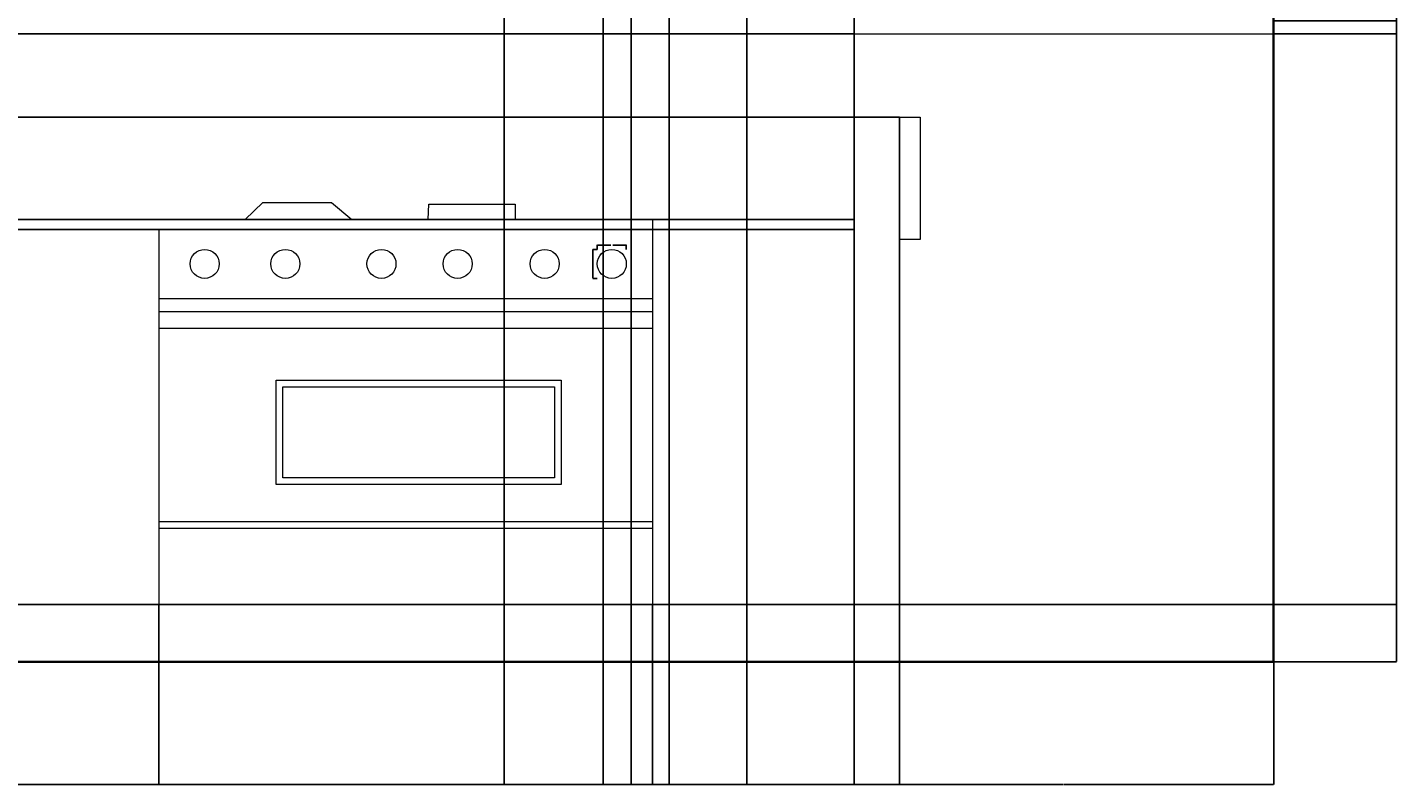
# Model space of a CAD drawing. Units: millimetres. Extents: x 4725 to 8727, y 2935 to 5260.
# Tile 2 of 3: x 6642 to 8727, y 2935 to 4087. Entities that reach past the tile are written whole.
import ezdxf

# ---------------------------------------------------------------- set-up
doc = ezdxf.new("R2010")
doc.units = ezdxf.units.MM
for name, color, linetype, lineweight in [('A-ANNO-DIMS', 2, 'Continuous', 18), ('A-CASE-CTOP', 7, 'Continuous', 25), ('A-ELEV', 7, 'Continuous', 35), ('A-EQPM', 4, 'Continuous', 18), ('A-FLOR-CASE', 8, 'Continuous', 25)]:
    doc.layers.add(name, color=color, linetype=linetype, lineweight=lineweight)
doc.styles.get("Standard").update_dxf_attribs({"font": 'arial.ttf'})
doc.dimstyles.get("Standard").update_dxf_attribs({"dimtxt": 0.18, "dimasz": 0.18, "dimexe": 0.18, "dimexo": 0.0625, "dimgap": 0.09, "dimtad": 0, "dimtih": 1, "dimtoh": 1, "dimdec": 4, "dimzin": 0, "dimdsep": 46, "dimtxsty": 'Standard', "dimcen": 0.09, "dimadec": 0, "dimazin": 0, "dimtfac": 1, "dimtdec": 4, "dimtofl": 0, "dimtmove": 0, "dimatfit": 3, "dimfxl": 1, "dimtolj": 1, "dimtzin": 0, "dimarcsym": 0})

# ---------------------------------------------------------------- blocks, each defined once
blk = doc.blocks.new('REFRIGERATOR-DOOR-PULL')
blk.add_lwpolyline([(0, 186.1), (31.3, 186.1), (31.3, 0), (0, 0)], close=True)
blk = doc.blocks.new('COOKER-CONTROL-KNOB')
blk.add_circle((22.1, 22.1), 22.1)
blk = doc.blocks.new('*D3')
at = {"layer": 'A-ANNO-DIMS', "color": 0, "lineweight": -2, "transparency": 16777216}
for p, q in [((7509.7, 3749.5), (7509.7, 3756.3)), ((7509.8, 3756.1), (7530.3, 3756.1)), ((7553.7, 3756.1), (7533.3, 3756.1)), ((7553.8, 3749.5), (7553.8, 3756.3))]:
    blk.add_line(p, q, dxfattribs=at)
at = {"layer": 'A-ANNO-DIMS', "color": 0, "transparency": 16777216}
for points in [[(7509.8, 3756.1), (7509.8, 3756), (7509.7, 3756.1)], [(7553.7, 3756.1), (7553.7, 3756), (7553.8, 3756.1)]]:
    blk.add_solid(points, dxfattribs=at)
at = {"layer": 'Defpoints', "color": 0, "transparency": 16777216}
for p in [(7553.8, 3756.1), (7509.7, 3749.4), (7553.8, 3749.4)]:
    blk.add_point(p, dxfattribs=at)
at = {"layer": 'A-ANNO-DIMS', "color": 0, "transparency": 16777216, "insert": (7531.8, 3756.1), "char_height": 0.18, "attachment_point": 5}
blk.add_mtext('\\A1;COOKER KNOB 44 TYP.', dxfattribs=at)
blk = doc.blocks.new('*D4')
at = {"layer": 'A-ANNO-DIMS', "color": 0, "lineweight": -2, "transparency": 16777216}
for p, q in [((7509.6, 3749.4), (7502.9, 3749.4)), ((7503, 3749.3), (7503, 3727.5)), ((7503, 3705.4), (7503, 3727.2)), ((7509.6, 3705.3), (7502.9, 3705.3))]:
    blk.add_line(p, q, dxfattribs=at)
at = {"layer": 'A-ANNO-DIMS', "color": 0, "transparency": 16777216}
for points in [[(7503, 3749.3), (7503.1, 3749.3), (7503, 3749.4)], [(7503, 3705.4), (7503.1, 3705.4), (7503, 3705.3)]]:
    blk.add_solid(points, dxfattribs=at)
at = {"layer": 'Defpoints', "color": 0, "transparency": 16777216}
for p in [(7503, 3749.4), (7509.7, 3749.4), (7509.7, 3705.3)]:
    blk.add_point(p, dxfattribs=at)
at = {"layer": 'A-ANNO-DIMS', "color": 0, "transparency": 16777216, "insert": (7503, 3727.4), "char_height": 0.18, "attachment_point": 5}
blk.add_mtext('\\A1;44 TYP.', dxfattribs=at)
blk = doc.blocks.new('*D10')
at = {"layer": 'A-ANNO-DIMS', "color": 0, "lineweight": -2, "transparency": 16777216}
for p, q in [((6031.8, 3209), (6031.8, 2934.7)), ((6841.9, 3209), (6841.9, 2934.7)), ((6032, 2934.8), (6436.5, 2934.8)), ((6841.8, 2934.8), (6437.3, 2934.8))]:
    blk.add_line(p, q, dxfattribs=at)
at = {"layer": 'A-ANNO-DIMS', "color": 0, "transparency": 16777216}
for points in [[(6032, 2934.9), (6032, 2934.8), (6031.8, 2934.8)], [(6841.8, 2934.9), (6841.8, 2934.8), (6841.9, 2934.8)]]:
    blk.add_solid(points, dxfattribs=at)
at = {"layer": 'Defpoints', "color": 0, "transparency": 16777216}
for p in [(6031.8, 3209), (6841.9, 3209), (6841.9, 2934.8)]:
    blk.add_point(p, dxfattribs=at)
at = {"layer": 'A-ANNO-DIMS', "color": 0, "transparency": 16777216, "insert": (6436.9, 2934.8), "char_height": 0.18, "attachment_point": 5}
blk.add_mtext('\\A1;810.2', dxfattribs=at)
blk = doc.blocks.new('*D11')
at = {"layer": 'A-ANNO-DIMS', "color": 0, "lineweight": -2, "transparency": 16777216}
for p, q in [((6841.9, 3209), (6841.9, 2934.7)), ((7593.8, 3209), (7593.8, 2934.7)), ((6842.1, 2934.8), (7217.5, 2934.8)), ((7593.6, 2934.8), (7218.3, 2934.8))]:
    blk.add_line(p, q, dxfattribs=at)
at = {"layer": 'A-ANNO-DIMS', "color": 0, "transparency": 16777216}
for points in [[(6842.1, 2934.9), (6842.1, 2934.8), (6841.9, 2934.8)], [(7593.6, 2934.9), (7593.6, 2934.8), (7593.8, 2934.8)]]:
    blk.add_solid(points, dxfattribs=at)
at = {"layer": 'Defpoints', "color": 0, "transparency": 16777216}
for p in [(6841.9, 3209), (7593.8, 3209), (7593.8, 2934.8)]:
    blk.add_point(p, dxfattribs=at)
at = {"layer": 'A-ANNO-DIMS', "color": 0, "transparency": 16777216, "insert": (7217.9, 2934.8), "char_height": 0.18, "attachment_point": 5}
blk.add_mtext('\\A1;751.9', dxfattribs=at)
blk = doc.blocks.new('*D12')
at = {"layer": 'A-ANNO-DIMS', "color": 0, "lineweight": -2, "transparency": 16777216}
for p, q in [((7593.8, 3209), (7593.8, 2934.7)), ((7900.9, 3121.6), (7900.9, 2934.7)), ((7594, 2934.8), (7746.9, 2934.8)), ((7900.7, 2934.8), (7747.8, 2934.8))]:
    blk.add_line(p, q, dxfattribs=at)
at = {"layer": 'A-ANNO-DIMS', "color": 0, "transparency": 16777216}
for points in [[(7594, 2934.9), (7594, 2934.8), (7593.8, 2934.8)], [(7900.7, 2934.9), (7900.7, 2934.8), (7900.9, 2934.8)]]:
    blk.add_solid(points, dxfattribs=at)
at = {"layer": 'Defpoints', "color": 0, "transparency": 16777216}
for p in [(7593.8, 3209), (7900.9, 3121.7), (7900.9, 2934.8)]:
    blk.add_point(p, dxfattribs=at)
at = {"layer": 'A-ANNO-DIMS', "color": 0, "transparency": 16777216, "insert": (7747.3, 2934.8), "char_height": 0.18, "attachment_point": 5}
blk.add_mtext('\\A1;307.04', dxfattribs=at)
blk = doc.blocks.new('*D13')
at = {"layer": 'A-ANNO-DIMS', "color": 0, "lineweight": -2, "transparency": 16777216}
for p, q in [((7900.9, 3121.6), (7900.9, 2934.7)), ((8539.6, 3121.6), (8539.6, 2934.7)), ((7901, 2934.8), (8219.8, 2934.8)), ((8539.4, 2934.8), (8220.6, 2934.8))]:
    blk.add_line(p, q, dxfattribs=at)
at = {"layer": 'A-ANNO-DIMS', "color": 0, "transparency": 16777216}
for points in [[(7901, 2934.9), (7901, 2934.8), (7900.9, 2934.8)], [(8539.4, 2934.9), (8539.4, 2934.8), (8539.6, 2934.8)]]:
    blk.add_solid(points, dxfattribs=at)
at = {"layer": 'Defpoints', "color": 0, "transparency": 16777216}
for p in [(7900.9, 3121.7), (8539.6, 3121.7), (8539.6, 2934.8)]:
    blk.add_point(p, dxfattribs=at)
at = {"layer": 'A-ANNO-DIMS', "color": 0, "transparency": 16777216, "insert": (8220.2, 2934.8), "char_height": 0.18, "attachment_point": 5}
blk.add_mtext('\\A1;638.7', dxfattribs=at)
blk = doc.blocks.new('*D21')
at = {"layer": 'A-ANNO-DIMS', "color": 0, "lineweight": -2, "transparency": 16777216}
for p, q in [((8539.6, 3209), (8726.6, 3209)), ((8726.4, 3208.8), (8726.4, 3165.5)), ((8726.4, 3121.9), (8726.4, 3165.2)), ((8539.6, 3121.7), (8726.6, 3121.7))]:
    blk.add_line(p, q, dxfattribs=at)
at = {"layer": 'A-ANNO-DIMS', "color": 0, "transparency": 16777216}
for points in [[(8726.4, 3208.8), (8726.4, 3208.8), (8726.4, 3209)], [(8726.4, 3121.9), (8726.4, 3121.9), (8726.4, 3121.7)]]:
    blk.add_solid(points, dxfattribs=at)
at = {"layer": 'Defpoints', "color": 0, "transparency": 16777216}
for p in [(8539.6, 3209), (8539.6, 3121.7), (8726.4, 3121.7)]:
    blk.add_point(p, dxfattribs=at)
at = {"layer": 'A-ANNO-DIMS', "color": 0, "transparency": 16777216, "insert": (8726.4, 3165.4), "char_height": 0.18, "attachment_point": 5}
blk.add_mtext('\\A1;87.33', dxfattribs=at)
blk = doc.blocks.new('*D26')
at = {"layer": 'A-ANNO-DIMS', "color": 0, "lineweight": -2, "transparency": 16777216}
for p, q in [((8539.6, 4077.4), (8726.6, 4077.4)), ((8726.4, 4077.2), (8726.4, 3643.4)), ((8726.4, 3209.2), (8726.4, 3643)), ((8539.6, 3209), (8726.6, 3209))]:
    blk.add_line(p, q, dxfattribs=at)
at = {"layer": 'A-ANNO-DIMS', "color": 0, "transparency": 16777216}
for points in [[(8726.4, 4077.2), (8726.4, 4077.2), (8726.4, 4077.4)], [(8726.4, 3209.2), (8726.4, 3209.2), (8726.4, 3209)]]:
    blk.add_solid(points, dxfattribs=at)
at = {"layer": 'Defpoints', "color": 0, "transparency": 16777216}
for p in [(8539.6, 4077.4), (8539.6, 3209), (8726.4, 3209)]:
    blk.add_point(p, dxfattribs=at)
at = {"layer": 'A-ANNO-DIMS', "color": 0, "transparency": 16777216, "insert": (8726.4, 3643.2), "char_height": 0.18, "attachment_point": 5}
blk.add_mtext('\\A1;868.4', dxfattribs=at)
blk = doc.blocks.new('*D27')
at = {"layer": 'A-ANNO-DIMS', "color": 0, "lineweight": -2, "transparency": 16777216}
for p, q in [((8539.6, 4097.4), (8726.6, 4097.4)), ((8726.4, 4097.2), (8726.4, 4087.6)), ((8726.4, 4077.6), (8726.4, 4087.2)), ((8539.6, 4077.4), (8726.6, 4077.4))]:
    blk.add_line(p, q, dxfattribs=at)
at = {"layer": 'A-ANNO-DIMS', "color": 0, "transparency": 16777216}
for points in [[(8726.4, 4097.2), (8726.4, 4097.2), (8726.4, 4097.4)], [(8726.4, 4077.6), (8726.4, 4077.6), (8726.4, 4077.4)]]:
    blk.add_solid(points, dxfattribs=at)
at = {"layer": 'Defpoints', "color": 0, "transparency": 16777216}
for p in [(8539.6, 4097.4), (8726.4, 4097.4), (8539.6, 4077.4)]:
    blk.add_point(p, dxfattribs=at)
at = {"layer": 'A-ANNO-DIMS', "color": 0, "transparency": 16777216, "insert": (8726.4, 4087.4), "char_height": 0.18, "attachment_point": 5}
blk.add_mtext('\\A1;20', dxfattribs=at)
blk = doc.blocks.new('*D32')
at = {"layer": 'A-ANNO-DIMS', "color": 0, "lineweight": -2, "transparency": 16777216}
for p, q in [((7367.7, 4364.8), (7367.7, 2934.7)), ((7518.4, 4364.8), (7518.4, 2934.7)), ((7367.8, 2934.8), (7442.6, 2934.8)), ((7518.2, 2934.8), (7443.5, 2934.8))]:
    blk.add_line(p, q, dxfattribs=at)
at = {"layer": 'A-ANNO-DIMS', "color": 0, "transparency": 16777216}
for points in [[(7367.8, 2934.9), (7367.8, 2934.8), (7367.7, 2934.8)], [(7518.2, 2934.9), (7518.2, 2934.8), (7518.4, 2934.8)]]:
    blk.add_solid(points, dxfattribs=at)
at = {"layer": 'Defpoints', "color": 0, "transparency": 16777216}
for p in [(7367.7, 4364.8), (7518.4, 4364.8), (7518.4, 2934.8)]:
    blk.add_point(p, dxfattribs=at)
at = {"layer": 'A-ANNO-DIMS', "color": 0, "transparency": 16777216, "insert": (7443, 2934.8), "char_height": 0.18, "attachment_point": 5}
blk.add_mtext('\\A1;150.77', dxfattribs=at)
blk = doc.blocks.new('*D33')
at = {"layer": 'A-ANNO-DIMS', "color": 0, "lineweight": -2, "transparency": 16777216}
for p, q in [((7518.4, 4364.8), (7518.4, 2934.7)), ((7561.3, 4334.1), (7561.3, 2934.7)), ((7518.6, 2934.8), (7539.4, 2934.8)), ((7561.2, 2934.8), (7540.3, 2934.8))]:
    blk.add_line(p, q, dxfattribs=at)
at = {"layer": 'A-ANNO-DIMS', "color": 0, "transparency": 16777216}
for points in [[(7518.6, 2934.9), (7518.6, 2934.8), (7518.4, 2934.8)], [(7561.2, 2934.9), (7561.2, 2934.8), (7561.3, 2934.8)]]:
    blk.add_solid(points, dxfattribs=at)
at = {"layer": 'Defpoints', "color": 0, "transparency": 16777216}
for p in [(7518.4, 4364.8), (7561.3, 4334.2), (7561.3, 2934.8)]:
    blk.add_point(p, dxfattribs=at)
at = {"layer": 'A-ANNO-DIMS', "color": 0, "transparency": 16777216, "insert": (7539.9, 2934.8), "char_height": 0.18, "attachment_point": 5}
blk.add_mtext('\\A1;42.905', dxfattribs=at)
blk = doc.blocks.new('*D34')
at = {"layer": 'A-ANNO-DIMS', "color": 0, "lineweight": -2, "transparency": 16777216}
for p, q in [((7619, 4410.2), (7619, 2934.7)), ((7737.5, 4410.2), (7737.5, 2934.7)), ((7619.2, 2934.8), (7677.8, 2934.8)), ((7737.4, 2934.8), (7678.7, 2934.8))]:
    blk.add_line(p, q, dxfattribs=at)
at = {"layer": 'A-ANNO-DIMS', "color": 0, "transparency": 16777216}
for points in [[(7619.2, 2934.9), (7619.2, 2934.8), (7619, 2934.8)], [(7737.4, 2934.9), (7737.4, 2934.8), (7737.5, 2934.8)]]:
    blk.add_solid(points, dxfattribs=at)
at = {"layer": 'Defpoints', "color": 0, "transparency": 16777216}
for p in [(7619, 4410.2), (7737.5, 4410.2), (7737.5, 2934.8)]:
    blk.add_point(p, dxfattribs=at)
at = {"layer": 'A-ANNO-DIMS', "color": 0, "transparency": 16777216, "insert": (7678.3, 2934.8), "char_height": 0.18, "attachment_point": 5}
blk.add_mtext('\\A1;118.53', dxfattribs=at)
blk = doc.blocks.new('*D35')
at = {"layer": 'A-ANNO-DIMS', "color": 0, "lineweight": -2, "transparency": 16777216}
for p, q in [((7737.5, 4410.2), (7737.5, 2934.7)), ((7900.9, 4334.1), (7900.9, 2934.7)), ((7737.7, 2934.8), (7818.7, 2934.8)), ((7900.7, 2934.8), (7819.7, 2934.8))]:
    blk.add_line(p, q, dxfattribs=at)
at = {"layer": 'A-ANNO-DIMS', "color": 0, "transparency": 16777216}
for points in [[(7737.7, 2934.9), (7737.7, 2934.8), (7737.5, 2934.8)], [(7900.7, 2934.9), (7900.7, 2934.8), (7900.9, 2934.8)]]:
    blk.add_solid(points, dxfattribs=at)
at = {"layer": 'Defpoints', "color": 0, "transparency": 16777216}
for p in [(7737.5, 4410.2), (7900.9, 4334.2), (7900.9, 2934.8)]:
    blk.add_point(p, dxfattribs=at)
at = {"layer": 'A-ANNO-DIMS', "color": 0, "transparency": 16777216, "insert": (7819.2, 2934.8), "char_height": 0.18, "attachment_point": 5}
blk.add_mtext('\\A1;163.32', dxfattribs=at)
blk = doc.blocks.new('*D41')
at = {"layer": 'A-ANNO-DIMS', "color": 0, "lineweight": -2, "transparency": 16777216}
for p, q in [((4912.4, 5073.1), (8726.6, 5073.1)), ((8726.4, 5072.9), (8726.4, 4097.6)), ((8726.4, 3121.9), (8726.4, 4097.2)), ((8539.6, 3121.7), (8726.6, 3121.7))]:
    blk.add_line(p, q, dxfattribs=at)
at = {"layer": 'A-ANNO-DIMS', "color": 0, "transparency": 16777216}
for points in [[(8726.4, 5072.9), (8726.4, 5072.9), (8726.4, 5073.1)], [(8726.4, 3121.9), (8726.4, 3121.9), (8726.4, 3121.7)]]:
    blk.add_solid(points, dxfattribs=at)
at = {"layer": 'Defpoints', "color": 0, "transparency": 16777216}
for p in [(4912.4, 5073.1), (8726.4, 5073.1), (8539.6, 3121.7)]:
    blk.add_point(p, dxfattribs=at)
at = {"layer": 'A-ANNO-DIMS', "color": 0, "transparency": 16777216, "insert": (8726.4, 4097.4), "char_height": 0.18, "attachment_point": 5}
blk.add_mtext('\\A1;1951.4', dxfattribs=at)
blk = doc.blocks.new('*D42')
at = {"layer": 'A-ANNO-DIMS', "color": 0, "lineweight": -2, "transparency": 16777216}
for p, q in [((7900.8, 4077.4), (4725.3, 4077.4)), ((4725.5, 4077.2), (4725.5, 4014.3)), ((4725.5, 3951), (4725.5, 4013.9)), ((7969.7, 3950.8), (4725.3, 3950.8))]:
    blk.add_line(p, q, dxfattribs=at)
at = {"layer": 'A-ANNO-DIMS', "color": 0, "transparency": 16777216}
for points in [[(4725.5, 4077.2), (4725.5, 4077.2), (4725.5, 4077.4)], [(4725.5, 3951), (4725.5, 3951), (4725.5, 3950.8)]]:
    blk.add_solid(points, dxfattribs=at)
at = {"layer": 'Defpoints', "color": 0, "transparency": 16777216}
for p in [(7900.9, 4077.4), (4725.5, 3950.8), (7969.8, 3950.8)]:
    blk.add_point(p, dxfattribs=at)
at = {"layer": 'A-ANNO-DIMS', "color": 0, "transparency": 16777216, "insert": (4725.5, 4014.1), "char_height": 0.18, "attachment_point": 5}
blk.add_mtext('\\A1;126.6', dxfattribs=at)
blk = doc.blocks.new('*D44')
at = {"layer": 'A-ANNO-DIMS', "color": 0, "lineweight": -2, "transparency": 16777216}
for p, q in [((7900.9, 4077.3), (7900.9, 2934.7)), ((7969.8, 3950.7), (7969.8, 2934.7)), ((7901, 2934.8), (7934.9, 2934.8)), ((7969.6, 2934.8), (7935.7, 2934.8))]:
    blk.add_line(p, q, dxfattribs=at)
at = {"layer": 'A-ANNO-DIMS', "color": 0, "transparency": 16777216}
for points in [[(7901, 2934.9), (7901, 2934.8), (7900.9, 2934.8)], [(7969.6, 2934.9), (7969.6, 2934.8), (7969.8, 2934.8)]]:
    blk.add_solid(points, dxfattribs=at)
at = {"layer": 'Defpoints', "color": 0, "transparency": 16777216}
for p in [(7900.9, 4077.4), (7969.8, 3950.8), (7969.8, 2934.8)]:
    blk.add_point(p, dxfattribs=at)
at = {"layer": 'A-ANNO-DIMS', "color": 0, "transparency": 16777216, "insert": (7935.3, 2934.8), "char_height": 0.18, "attachment_point": 5}
blk.add_mtext('\\A1;68.91', dxfattribs=at)

msp = doc.modelspace()

# ---------------------------------------------------------------- linework, layer by layer
at = {"layer": 'A-CASE-CTOP'}
for p, q in [((7900.8562, 3794.7145), (4912.3658, 3794.7145)), ((7900.8562, 3779.7145), (4912.3658, 3779.7145))]:
    msp.add_line(p, q, dxfattribs=at)
at = {"layer": 'A-ELEV'}
for p, q in [((8539.5662, 5073.1177), (8539.5662, 3121.6884)), ((8539.5662, 3121.6884), (4912.3658, 3121.6884))]:
    msp.add_line(p, q, dxfattribs=at)
at = {"layer": 'A-EQPM'}
for p, q in [((7900.8562, 4077.4031), (8539.5662, 4077.4031)), ((6973.3154, 3794.7145), (7000.1563, 3820.9774)), ((7000.1563, 3820.9774), (7104.9228, 3820.9774)), ((7104.9228, 3820.9774), (7136.0929, 3794.7145)), ((7252.1152, 3794.7145), (7252.9811, 3818.3822)), ((7252.9811, 3818.3822), (7384.5885, 3818.3822)), ((7384.5885, 3818.3822), (7384.5885, 3794.7145)), ((7593.8125, 3794.7145), (7593.8125, 3209.0157)), ((6841.9423, 3779.7145), (6841.9423, 3209.0157)), ((7593.8125, 3674.2392), (6841.9423, 3674.2392)), ((7593.8125, 3654.2392), (6841.9423, 3654.2392)), ((7593.8125, 3629.2392), (6841.9423, 3629.2392)), ((6841.9423, 3335.1852), (7593.8125, 3335.1852)), ((6841.9423, 3325.1852), (7593.8125, 3325.1852))]:
    msp.add_line(p, q, dxfattribs=at)
for points in [[(7020.8517, 3550.3993), (7454.4116, 3550.3993), (7454.4116, 3391.7479), (7020.8517, 3391.7479)], [(7030.8517, 3540.3993), (7444.4116, 3540.3993), (7444.4116, 3401.7479), (7030.8517, 3401.7479)]]:
    msp.add_lwpolyline(points, close=True, dxfattribs=at)
at = {"layer": 'A-FLOR-CASE'}
for p, q in [((7900.8562, 5073.1177), (7900.8562, 3121.6884)), ((8539.5662, 3209.0157), (4912.3658, 3209.0157))]:
    msp.add_line(p, q, dxfattribs=at)

# ---------------------------------------------------------------- block references
at = {"layer": 'A-EQPM'}
for name, p in [('REFRIGERATOR-DOOR-PULL', (7969.768, 3764.7134)), ('COOKER-CONTROL-KNOB', (6889.7, 3705.265)), ('COOKER-CONTROL-KNOB', (7012.588, 3705.265)), ('COOKER-CONTROL-KNOB', (7158.949, 3705.265)), ('COOKER-CONTROL-KNOB', (7274.9331, 3705.265)), ('COOKER-CONTROL-KNOB', (7407.4865, 3705.265)), ('COOKER-CONTROL-KNOB', (7509.663, 3705.265))]:
    msp.add_blockref(name, p, dxfattribs=at)

# ---------------------------------------------------------------- dimensions: what is measured, and where the dimension line sits
at = {"layer": 'A-ANNO-DIMS'}
for base, p1, p2, override, picture, middle in [((8726.4162, 5073.1177), (8539.5662, 3121.6884), (4912.3658, 5073.1177), {"dimdec": 1, "dimlfac": 1, "dimrnd": 0, "dimzin": 0, "dimdsep": 46, "dimlunit": 2}, '*D41', (8726.4162, 4097.4031)), ((8726.4162, 4097.4031), (8539.5662, 4077.4031), (8539.5662, 4097.4031), {"dimdec": 0, "dimlfac": 1, "dimrnd": 0, "dimzin": 0, "dimdsep": 46, "dimlunit": 2}, '*D27', (8726.4162, 4087.4031)), ((4725.5158, 3950.7955), (7900.8562, 4077.4031), (7969.7678, 3950.7955), {"dimdec": 1, "dimlfac": 1, "dimrnd": 0, "dimzin": 0, "dimdsep": 46, "dimlunit": 2}, '*D42', (4725.5158, 4014.0993)), ((8726.4162, 3209.0157), (8539.5662, 4077.4031), (8539.5662, 3209.0157), {"dimdec": 1, "dimlfac": 1, "dimrnd": 0, "dimzin": 0, "dimdsep": 46, "dimlunit": 2}, '*D26', (8726.4162, 3643.2094)), ((8726.4162, 3121.6884), (8539.5662, 3209.0157), (8539.5662, 3121.6884), {"dimdec": 2, "dimlfac": 1, "dimrnd": 0, "dimzin": 0, "dimdsep": 46, "dimlunit": 2}, '*D21', (8726.4162, 3165.3521))]:
    dim = msp.add_linear_dim(base=base, p1=p1, p2=p2, angle=90, dimstyle='Standard', override=override, dxfattribs=at)
    dim.commit()
    dim.dimension.update_dxf_attribs({"geometry": picture, "text_midpoint": middle})
for base, p1, p2, override, picture, middle in [((7737.5372, 2934.8384), (7619.0046, 4410.2347), (7737.5372, 4410.2347), {"dimdec": 2, "dimlfac": 1, "dimrnd": 0, "dimzin": 0, "dimdsep": 46, "dimlunit": 2}, '*D34', (7678.2709, 2934.8384)), ((7900.8562, 2934.8384), (7737.5372, 4410.2347), (7900.8562, 4334.1944), {"dimdec": 2, "dimlfac": 1, "dimrnd": 0, "dimzin": 0, "dimdsep": 46, "dimlunit": 2}, '*D35', (7819.1967, 2934.8384)), ((7518.4266, 2934.8384), (7367.6547, 4364.8232), (7518.4266, 4364.8232), {"dimdec": 2, "dimlfac": 1, "dimrnd": 0, "dimzin": 0, "dimdsep": 46, "dimlunit": 2}, '*D32', (7443.0406, 2934.8384)), ((7561.3315, 2934.8384), (7518.4266, 4364.8232), (7561.3315, 4334.1944), {"dimdec": 3, "dimlfac": 1, "dimrnd": 0, "dimzin": 0, "dimdsep": 46, "dimlunit": 2}, '*D33', (7539.879, 2934.8384)), ((7969.7678, 2934.8384), (7900.8562, 4077.4031), (7969.7678, 3950.7955), {"dimdec": 2, "dimlfac": 1, "dimrnd": 0, "dimzin": 0, "dimdsep": 46, "dimlunit": 2}, '*D44', (7935.312, 2934.8384)), ((6841.9423, 2934.8384), (6031.7891, 3209.0157), (6841.9423, 3209.0157), {"dimdec": 1, "dimlfac": 1, "dimrnd": 0, "dimzin": 0, "dimdsep": 46, "dimlunit": 2}, '*D10', (6436.8657, 2934.8384)), ((7593.8125, 2934.8384), (6841.9423, 3209.0157), (7593.8125, 3209.0157), {"dimdec": 1, "dimlfac": 1, "dimrnd": 0, "dimzin": 0, "dimdsep": 46, "dimlunit": 2}, '*D11', (7217.8774, 2934.8384)), ((7900.8562, 2934.8384), (7593.8125, 3209.0157), (7900.8562, 3121.6884), {"dimdec": 2, "dimlfac": 1, "dimrnd": 0, "dimzin": 0, "dimdsep": 46, "dimlunit": 2}, '*D12', (7747.3344, 2934.8384)), ((8539.5662, 2934.8384), (7900.8562, 3121.6884), (8539.5662, 3121.6884), {"dimdec": 1, "dimlfac": 1, "dimrnd": 0, "dimzin": 0, "dimdsep": 46, "dimlunit": 2}, '*D13', (8220.2112, 2934.8384))]:
    dim = msp.add_linear_dim(base=base, p1=p1, p2=p2, dimstyle='Standard', override=override, dxfattribs=at)
    dim.commit()
    dim.dimension.update_dxf_attribs({"geometry": picture, "text_midpoint": middle})
dim = msp.add_linear_dim(base=(7553.8474, 3756.0766), p1=(7509.663, 3749.449), p2=(7553.8474, 3749.449), text='COOKER KNOB <> TYP.', dimstyle='Standard', override={"dimdec": 0, "dimlfac": 1, "dimrnd": 0, "dimzin": 0, "dimdsep": 46, "dimlunit": 2}, dxfattribs=at)
dim.commit()
dim.dimension.update_dxf_attribs({"geometry": '*D3', "text_midpoint": (7531.7552, 3756.0766)})
dim = msp.add_linear_dim(base=(7503.0353, 3749.449), p1=(7509.663, 3705.2645), p2=(7509.663, 3749.449), angle=90, text='<> TYP.', dimstyle='Standard', override={"dimdec": 0, "dimlfac": 1, "dimrnd": 0, "dimzin": 0, "dimdsep": 46, "dimlunit": 2}, dxfattribs=at)
dim.commit()
dim.dimension.update_dxf_attribs({"geometry": '*D4', "text_midpoint": (7503.0353, 3727.3567)})

doc.saveas('drawing.dxf')
